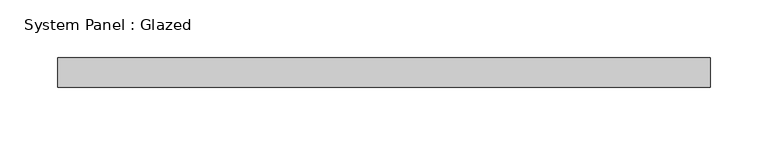
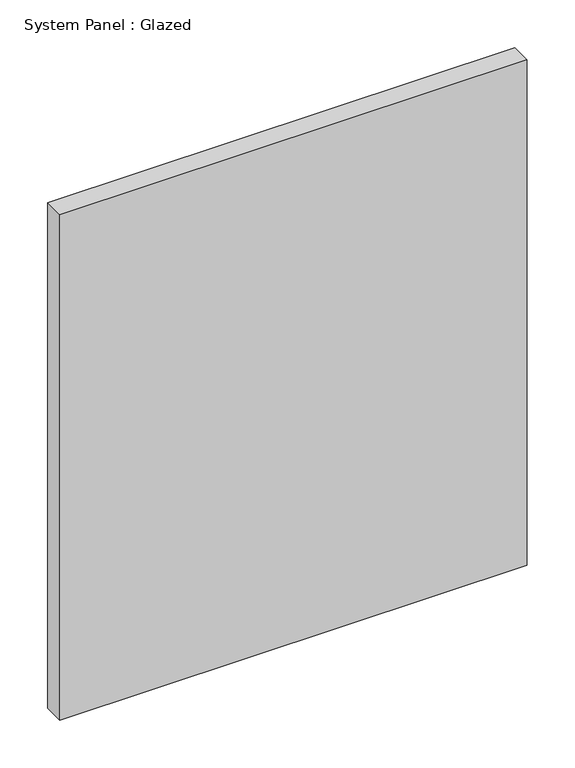
"""IFC4 building model written with IfcOpenShell, lengths in millimetres: plate geometry, System Panel : Glazed."""

from ifc_helpers import new_model, si_unit, origin, origin_with_axes, place, context, project, spatial, polyline, outline, extrude, source, transform, mapped, element, save


def system_panel_glazed_748c8dd9(model_context):
    return source(origin(), model_context, "Body", "SweptSolid", [
        extrude(outline(polyline([(282.575, 19.05), (-282.575, 19.05), (-282.575, 44.45), (282.575, 44.45), (282.575, 19.05)])), origin_with_axes(), (0.0, 0.0, 1.0), 646.1658453),
    ])


if __name__ == "__main__":
    model = new_model("IFC4")
    model_context = context("Model", 3, world=origin())
    ifc_project = project(units=[si_unit("LENGTHUNIT", "METRE", prefix="MILLI")], contexts=[model_context])
    site = spatial("IfcSite", under=ifc_project)
    building = spatial("IfcBuilding", under=site)
    placement = place(None, origin())
    system_panel_glazed_shape = system_panel_glazed_748c8dd9(model_context)
    element("IfcPlate", 1, ObjectType="System Panel : Glazed", at=placement, inside=building, context=model_context, shape_type="MappedRepresentation", body=[
        mapped(system_panel_glazed_shape, transform((0.0, 0.0, 0.0), x_axis=(1.0, 0.0, 0.0), y_axis=(0.0, 1.0, 0.0), z_axis=(0.0, 0.0, 1.0))),
    ])
    save(model, "model.ifc")

# Revit data of these elements
# Type "System Panel : Glazed"
#   Construction Type Id = "GSP4R"
#   Analytic Construction = "1/8 in Pilkington single glazing"
#   Visual Light Transmittance = 0.9
#   Solar Heat Gain Coefficient = 0.86
#   Heat Transfer Coefficient (U) = 1.18115 BTU/(h·ft²·°F)
#   Define Thermal Properties by = 1
# Element 1 (IfcPlate, "System Panel : Glazed")
#   Materials on its faces: "Glass"
# Materials
#   "Glass": class "Glass", colour RGB 0 128 192, transparency 0.75, Description = "Soda Lime Glass", Cost = 0
